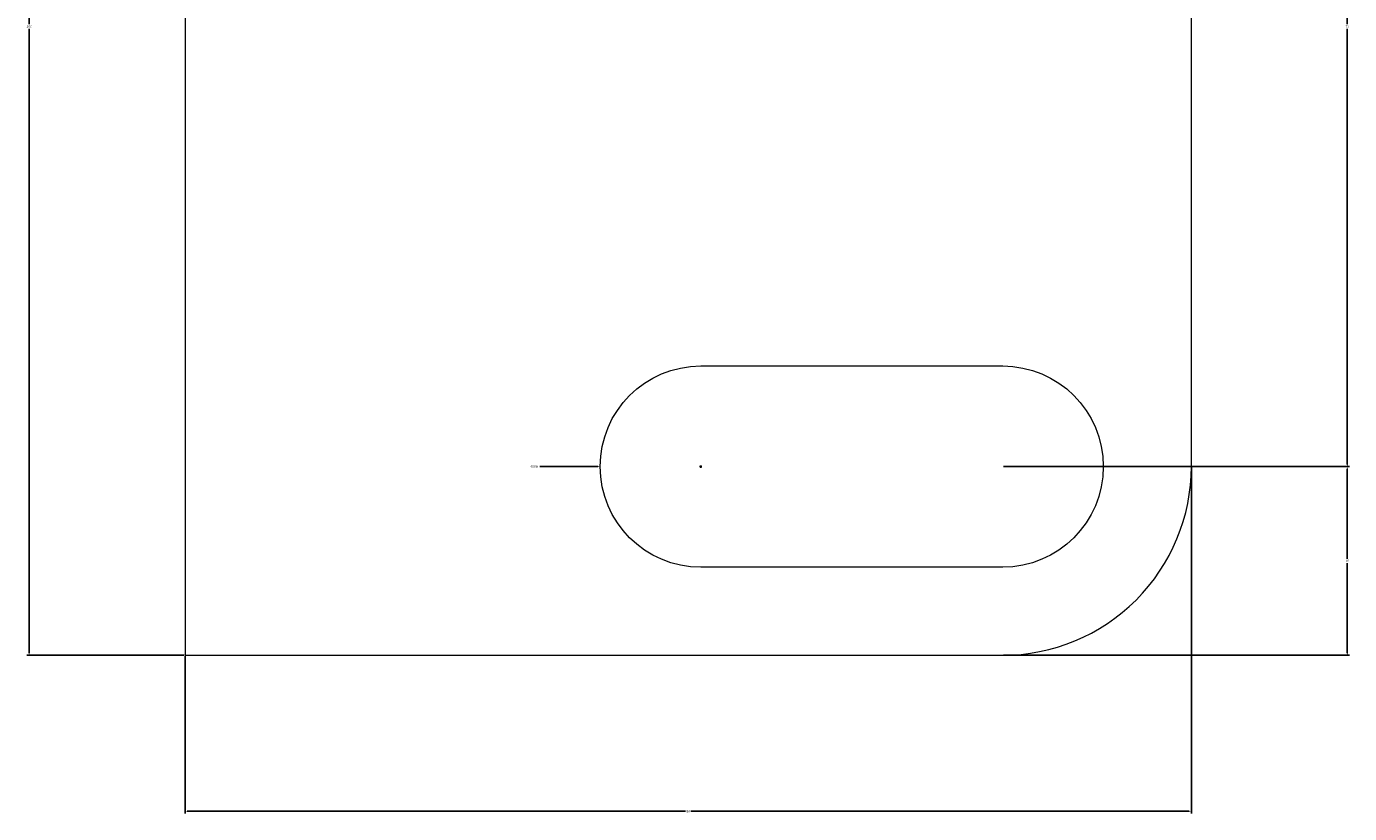
# Model space of a CAD drawing. Units: millimetres. Extents: x 2815 to 2920, y 1079 to 1204.
# Tile 1 of 2: x 2815 to 2920, y 1079 to 1141. Entities that reach past the tile are written whole.
import ezdxf

# ---------------------------------------------------------------- set-up
doc = ezdxf.new("R2010")
doc.units = ezdxf.units.MM
doc.layers.add('M-CONS', color=7, linetype='Continuous', lineweight=18)
doc.layers.add('M-DIMS', color=2, linetype='Continuous', lineweight=18)
doc.styles.get("Standard").update_dxf_attribs({"font": 'arial.ttf'})
doc.dimstyles.get("Standard").update_dxf_attribs({"dimtxt": 0.18, "dimasz": 0.18, "dimexe": 0.18, "dimexo": 0.0625, "dimgap": 0.09, "dimtad": 0, "dimtih": 1, "dimtoh": 1, "dimdec": 4, "dimzin": 0, "dimdsep": 46, "dimtxsty": 'Standard', "dimcen": 0.09, "dimadec": 0, "dimazin": 0, "dimtfac": 1, "dimtdec": 4, "dimtofl": 0, "dimtmove": 0, "dimatfit": 3, "dimfxl": 1, "dimtolj": 1, "dimtzin": 0, "dimarcsym": 0})

# ---------------------------------------------------------------- blocks, each defined once
blk = doc.blocks.new('*D1')
at = {"layer": 'Defpoints', "color": 0, "transparency": 16777216}
for p in [(2907.45, 1106.18), (2827.45, 1091.18), (2907.45, 1078.78)]:
    blk.add_point(p, dxfattribs=at)
at = {"layer": 'M-DIMS', "color": 0, "lineweight": -2, "transparency": 16777216}
for p, q in [((2907.45, 1106.11), (2907.45, 1078.6)), ((2827.45, 1091.11), (2827.45, 1078.6)), ((2827.63, 1078.78), (2867.23, 1078.78)), ((2907.27, 1078.78), (2867.66, 1078.78))]:
    blk.add_line(p, q, dxfattribs=at)
at = {"layer": 'M-DIMS', "color": 0, "transparency": 16777216}
for points in [[(2827.63, 1078.81), (2827.63, 1078.75), (2827.45, 1078.78)], [(2907.27, 1078.81), (2907.27, 1078.75), (2907.45, 1078.78)]]:
    blk.add_solid(points, dxfattribs=at)
at = {"layer": 'M-DIMS', "color": 0, "transparency": 16777216, "insert": (2867.45, 1078.78), "char_height": 0.18, "attachment_point": 5}
blk.add_mtext('\\A1;80', dxfattribs=at)
blk = doc.blocks.new('*D2')
at = {"layer": 'Defpoints', "color": 0, "transparency": 16777216}
for p in [(2815.05, 1191.18), (2827.45, 1191.18), (2827.45, 1091.18)]:
    blk.add_point(p, dxfattribs=at)
at = {"layer": 'M-DIMS', "color": 0, "lineweight": -2, "transparency": 16777216}
for p, q in [((2827.38, 1191.18), (2814.87, 1191.18)), ((2815.05, 1191), (2815.05, 1141.36)), ((2815.05, 1091.36), (2815.05, 1140.99)), ((2827.38, 1091.18), (2814.87, 1091.18))]:
    blk.add_line(p, q, dxfattribs=at)
at = {"layer": 'M-DIMS', "color": 0, "transparency": 16777216}
for points in [[(2815.02, 1191), (2815.08, 1191), (2815.05, 1191.18)], [(2815.02, 1091.36), (2815.08, 1091.36), (2815.05, 1091.18)]]:
    blk.add_solid(points, dxfattribs=at)
at = {"layer": 'M-DIMS', "color": 0, "transparency": 16777216, "insert": (2815.05, 1141.18), "char_height": 0.18, "attachment_point": 5}
blk.add_mtext('\\A1;100', dxfattribs=at)
blk = doc.blocks.new('*D5')
at = {"layer": 'Defpoints', "color": 0, "transparency": 16777216}
for p in [(2892.45, 1106.18), (2919.85, 1106.18), (2892.45, 1091.18)]:
    blk.add_point(p, dxfattribs=at)
at = {"layer": 'M-DIMS', "color": 0, "lineweight": -2, "transparency": 16777216}
for p, q in [((2892.51, 1106.18), (2920.03, 1106.18)), ((2919.85, 1106), (2919.85, 1098.86)), ((2919.85, 1091.36), (2919.85, 1098.49)), ((2892.51, 1091.18), (2920.03, 1091.18))]:
    blk.add_line(p, q, dxfattribs=at)
at = {"layer": 'M-DIMS', "color": 0, "transparency": 16777216}
for points in [[(2919.82, 1106), (2919.88, 1106), (2919.85, 1106.18)], [(2919.82, 1091.36), (2919.88, 1091.36), (2919.85, 1091.18)]]:
    blk.add_solid(points, dxfattribs=at)
at = {"layer": 'M-DIMS', "color": 0, "transparency": 16777216, "insert": (2919.85, 1098.68), "char_height": 0.18, "attachment_point": 5}
blk.add_mtext('\\A1;15', dxfattribs=at)
blk = doc.blocks.new('*D6')
at = {"layer": 'Defpoints', "color": 0, "transparency": 16777216}
for p in [(2892.45, 1176.18), (2919.85, 1176.18), (2892.45, 1106.18)]:
    blk.add_point(p, dxfattribs=at)
at = {"layer": 'M-DIMS', "color": 0, "lineweight": -2, "transparency": 16777216}
for p, q in [((2892.51, 1176.18), (2920.03, 1176.18)), ((2919.85, 1176), (2919.85, 1141.36)), ((2919.85, 1106.36), (2919.85, 1140.99)), ((2892.51, 1106.18), (2920.03, 1106.18))]:
    blk.add_line(p, q, dxfattribs=at)
at = {"layer": 'M-DIMS', "color": 0, "transparency": 16777216}
for points in [[(2919.82, 1176), (2919.88, 1176), (2919.85, 1176.18)], [(2919.82, 1106.36), (2919.88, 1106.36), (2919.85, 1106.18)]]:
    blk.add_solid(points, dxfattribs=at)
at = {"layer": 'M-DIMS', "color": 0, "transparency": 16777216, "insert": (2919.85, 1141.18), "char_height": 0.18, "attachment_point": 5}
blk.add_mtext('\\A1;70', dxfattribs=at)
blk = doc.blocks.new('*D8')
at = {"layer": 'Defpoints', "color": 0, "transparency": 16777216}
for p in [(2860.45, 1106.18), (2868.45, 1106.18)]:
    blk.add_point(p, dxfattribs=at)
at = {"layer": 'M-DIMS', "color": 0, "lineweight": -2, "transparency": 16777216}
for p, q in [((2855.65, 1106.18), (2860.27, 1106.18)), ((2868.36, 1106.18), (2868.54, 1106.18)), ((2868.45, 1106.09), (2868.45, 1106.27))]:
    blk.add_line(p, q, dxfattribs=at)
at = {"layer": 'M-DIMS', "color": 0, "transparency": 16777216}
blk.add_solid([(2860.27, 1106.21), (2860.27, 1106.15), (2860.45, 1106.18)], dxfattribs=at)
at = {"layer": 'M-DIMS', "color": 0, "transparency": 16777216, "insert": (2855.21, 1106.18), "char_height": 0.18, "attachment_point": 5}
blk.add_mtext('\\A1;4X R8', dxfattribs=at)

msp = doc.modelspace()

# ---------------------------------------------------------------- linework, layer by layer
at = {"layer": 'M-CONS'}
for points in [[(2907.45, 1176.18, 0.414214), (2892.45, 1191.18), (2827.45, 1191.18), (2827.45, 1091.18), (2892.45, 1091.18, 0.414214), (2907.45, 1106.18)], [(2868.45, 1114.18), (2892.45, 1114.18, -1), (2892.45, 1098.18), (2868.45, 1098.18, -1)]]:
    msp.add_lwpolyline(points, format="xyb", close=True, dxfattribs=at)

# ---------------------------------------------------------------- dimensions: what is measured, and where the dimension line sits
at = {"layer": 'M-DIMS'}
for base, p1, p2, picture, middle in [((2815.05, 1191.18), (2827.45, 1091.18), (2827.45, 1191.18), '*D2', (2815.05, 1141.18)), ((2919.85, 1176.18), (2892.45, 1106.18), (2892.45, 1176.18), '*D6', (2919.85, 1141.18)), ((2919.85, 1106.18), (2892.45, 1091.18), (2892.45, 1106.18), '*D5', (2919.85, 1098.68))]:
    dim = msp.add_linear_dim(base=base, p1=p1, p2=p2, angle=90, dimstyle='Standard', override={"dimdec": 0, "dimlfac": 1, "dimrnd": 0, "dimzin": 0, "dimdsep": 46, "dimlunit": 2}, dxfattribs=at)
    dim.commit()
    dim.dimension.update_dxf_attribs({"geometry": picture, "text_midpoint": middle})
dim = msp.add_linear_dim(base=(2907.45, 1078.78), p1=(2827.45, 1091.18), p2=(2907.45, 1106.18), dimstyle='Standard', override={"dimdec": 0, "dimlfac": 1, "dimrnd": 0, "dimzin": 0, "dimdsep": 46, "dimlunit": 2}, dxfattribs=at)
dim.commit()
dim.dimension.update_dxf_attribs({"geometry": '*D1', "text_midpoint": (2867.45, 1078.78)})
dim = msp.add_radius_dim(center=(2868.45, 1106.18), mpoint=(2860.45, 1106.18), text='4X <>', dimstyle='Standard', override={"dimdec": 0, "dimlfac": 1, "dimrnd": 0, "dimzin": 0, "dimdsep": 46, "dimlunit": 2}, dxfattribs=at)
dim.commit()
dim.dimension.update_dxf_attribs({"geometry": '*D8', "text_midpoint": (2855.65, 1106.18), "dimtype": 164})

doc.saveas('drawing.dxf')
